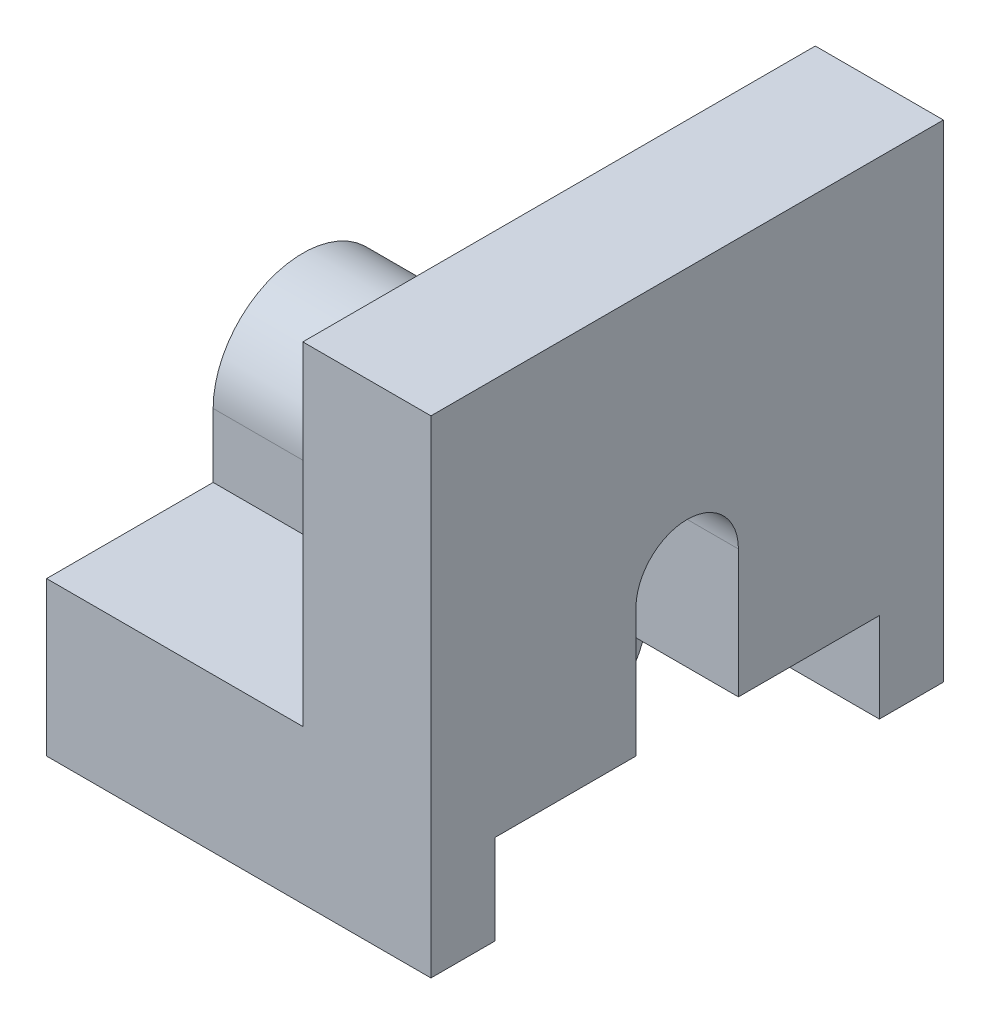
ISO-10303-21;
HEADER;
FILE_DESCRIPTION(('STEP AP214'),'2;1');
FILE_NAME('part.step','',(''),(''),'','','');
FILE_SCHEMA(('AUTOMOTIVE_DESIGN { 1 0 10303 214 1 1 1 1 }'));
ENDSEC;
DATA;
#1=APPLICATION_CONTEXT('core data for automotive mechanical design processes');
#2=APPLICATION_PROTOCOL_DEFINITION('international standard','automotive_design',2000,#1);
#3=PRODUCT_CONTEXT('',#1,'mechanical');
#4=PRODUCT('Part','Part','',(#3));
#5=PRODUCT_RELATED_PRODUCT_CATEGORY('part','',(#4));
#6=PRODUCT_DEFINITION_FORMATION('','',#4);
#7=PRODUCT_DEFINITION_CONTEXT('part definition',#1,'design');
#8=PRODUCT_DEFINITION('design','',#6,#7);
#9=PRODUCT_DEFINITION_SHAPE('','',#8);
#10=(LENGTH_UNIT() NAMED_UNIT(*) SI_UNIT(.MILLI.,.METRE.));
#11=(NAMED_UNIT(*) PLANE_ANGLE_UNIT() SI_UNIT($,.RADIAN.));
#12=(NAMED_UNIT(*) SI_UNIT($,.STERADIAN.) SOLID_ANGLE_UNIT());
#13=UNCERTAINTY_MEASURE_WITH_UNIT(LENGTH_MEASURE(1.E-05),#10,'distance_accuracy_value','');
#14=(GEOMETRIC_REPRESENTATION_CONTEXT(3) GLOBAL_UNCERTAINTY_ASSIGNED_CONTEXT((#13)) GLOBAL_UNIT_ASSIGNED_CONTEXT((#10,
#11,#12)) REPRESENTATION_CONTEXT('',''));
#15=CARTESIAN_POINT('',(0.,0.,0.));
#16=DIRECTION('',(0.,0.,1.));
#17=DIRECTION('',(1.,0.,0.));
#18=AXIS2_PLACEMENT_3D('',#15,#16,#17);
#19=CARTESIAN_POINT('',(20.,12.,40.));
#20=DIRECTION('',(1.,0.,0.));
#21=DIRECTION('',(0.,0.,-1.));
#22=AXIS2_PLACEMENT_3D('',#19,#20,#21);
#23=PLANE('',#22);
#24=DIRECTION('',(0.,-1.,0.));
#25=VECTOR('',#24,1.);
#26=CARTESIAN_POINT('',(20.,12.,17.5));
#27=LINE('',#26,#25);
#28=CARTESIAN_POINT('',(20.,38.,17.5));
#29=VERTEX_POINT('',#28);
#30=CARTESIAN_POINT('',(20.,23.538348415311,17.5));
#31=VERTEX_POINT('',#30);
#32=EDGE_CURVE('E53',#29,#31,#27,.T.);
#33=ORIENTED_EDGE('',*,*,#32,.F.);
#34=DIRECTION('',(0.,0.,-1.));
#35=VECTOR('',#34,1.);
#36=CARTESIAN_POINT('',(20.,38.,40.));
#37=LINE('',#36,#35);
#38=CARTESIAN_POINT('',(20.,38.,0.));
#39=VERTEX_POINT('',#38);
#40=EDGE_CURVE('E219',#29,#39,#37,.T.);
#41=ORIENTED_EDGE('',*,*,#40,.T.);
#42=DIRECTION('',(0.,-1.,0.));
#43=VECTOR('',#42,1.);
#44=CARTESIAN_POINT('',(20.,12.,0.));
#45=LINE('',#44,#43);
#46=CARTESIAN_POINT('',(20.,12.,0.));
#47=VERTEX_POINT('',#46);
#48=EDGE_CURVE('E283',#39,#47,#45,.T.);
#49=ORIENTED_EDGE('',*,*,#48,.T.);
#50=DIRECTION('',(0.,0.,-1.));
#51=VECTOR('',#50,1.);
#52=CARTESIAN_POINT('',(20.,12.,40.));
#53=LINE('',#52,#51);
#54=CARTESIAN_POINT('',(20.,12.,13.));
#55=VERTEX_POINT('',#54);
#56=EDGE_CURVE('E234',#55,#47,#53,.T.);
#57=ORIENTED_EDGE('',*,*,#56,.F.);
#58=DIRECTION('',(0.,-1.,0.));
#59=VECTOR('',#58,1.);
#60=CARTESIAN_POINT('',(20.,7.00000000000001,13.));
#61=LINE('',#60,#59);
#62=CARTESIAN_POINT('',(20.,17.,13.));
#63=VERTEX_POINT('',#62);
#64=EDGE_CURVE('E336',#63,#55,#61,.T.);
#65=ORIENTED_EDGE('',*,*,#64,.F.);
#66=CARTESIAN_POINT('',(20.,17.,20.));
#67=DIRECTION('',(-1.,0.,0.));
#68=DIRECTION('',(0.,0.,1.));
#69=AXIS2_PLACEMENT_3D('',#66,#67,#68);
#70=CIRCLE('',#69,7.);
#71=EDGE_CURVE('E63',#31,#63,#70,.T.);
#72=ORIENTED_EDGE('',*,*,#71,.F.);
#73=EDGE_LOOP('',(#33,#41,#49,#57,#65,#72));
#74=FACE_BOUND('',#73,.T.);
#75=ADVANCED_FACE('F39',(#74),#23,.F.);
#76=CARTESIAN_POINT('',(30.,7.,0.));
#77=DIRECTION('',(0.,1.,0.));
#78=DIRECTION('',(0.,0.,1.));
#79=AXIS2_PLACEMENT_3D('',#76,#77,#78);
#80=PLANE('',#79);
#81=DIRECTION('',(0.,0.,1.));
#82=VECTOR('',#81,1.);
#83=CARTESIAN_POINT('',(20.,7.,0.));
#84=LINE('',#83,#82);
#85=CARTESIAN_POINT('',(20.,7.,24.));
#86=VERTEX_POINT('',#85);
#87=CARTESIAN_POINT('',(20.,7.,27.));
#88=VERTEX_POINT('',#87);
#89=EDGE_CURVE('E43',#86,#88,#84,.T.);
#90=ORIENTED_EDGE('',*,*,#89,.F.);
#91=DIRECTION('',(-1.,0.,0.));
#92=VECTOR('',#91,1.);
#93=CARTESIAN_POINT('',(30.,7.,24.));
#94=LINE('',#93,#92);
#95=CARTESIAN_POINT('',(30.,7.,24.));
#96=VERTEX_POINT('',#95);
#97=EDGE_CURVE('E383',#96,#86,#94,.T.);
#98=ORIENTED_EDGE('',*,*,#97,.F.);
#99=DIRECTION('',(0.,0.,-1.));
#100=VECTOR('',#99,1.);
#101=CARTESIAN_POINT('',(30.,7.,0.));
#102=LINE('',#101,#100);
#103=CARTESIAN_POINT('',(30.,7.,35.));
#104=VERTEX_POINT('',#103);
#105=EDGE_CURVE('E322',#104,#96,#102,.T.);
#106=ORIENTED_EDGE('',*,*,#105,.F.);
#107=DIRECTION('',(-1.,0.,0.));
#108=VECTOR('',#107,1.);
#109=CARTESIAN_POINT('',(30.,7.,35.));
#110=LINE('',#109,#108);
#111=CARTESIAN_POINT('',(0.,7.,35.));
#112=VERTEX_POINT('',#111);
#113=EDGE_CURVE('E301',#104,#112,#110,.T.);
#114=ORIENTED_EDGE('',*,*,#113,.T.);
#115=DIRECTION('',(0.,0.,-1.));
#116=VECTOR('',#115,1.);
#117=CARTESIAN_POINT('',(0.,7.,0.));
#118=LINE('',#117,#116);
#119=CARTESIAN_POINT('',(0.,7.,27.));
#120=VERTEX_POINT('',#119);
#121=EDGE_CURVE('E314',#112,#120,#118,.T.);
#122=ORIENTED_EDGE('',*,*,#121,.T.);
#123=DIRECTION('',(-1.,0.,0.));
#124=VECTOR('',#123,1.);
#125=CARTESIAN_POINT('',(20.,7.00000000000001,27.));
#126=LINE('',#125,#124);
#127=EDGE_CURVE('E331',#88,#120,#126,.T.);
#128=ORIENTED_EDGE('',*,*,#127,.F.);
#129=EDGE_LOOP('',(#90,#98,#106,#114,#122,#128));
#130=FACE_BOUND('',#129,.T.);
#131=ADVANCED_FACE('F444',(#130),#80,.F.);
#132=CARTESIAN_POINT('',(30.,6.99999999999997,16.));
#133=VERTEX_POINT('',#132);
#134=CARTESIAN_POINT('',(30.,7.,5.));
#135=VERTEX_POINT('',#134);
#136=EDGE_CURVE('E330',#133,#135,#102,.T.);
#137=ORIENTED_EDGE('',*,*,#136,.F.);
#138=DIRECTION('',(-1.,0.,0.));
#139=VECTOR('',#138,1.);
#140=CARTESIAN_POINT('',(30.,6.99999999999997,16.));
#141=LINE('',#140,#139);
#142=CARTESIAN_POINT('',(20.,6.99999999999997,16.));
#143=VERTEX_POINT('',#142);
#144=EDGE_CURVE('E387',#133,#143,#141,.T.);
#145=ORIENTED_EDGE('',*,*,#144,.T.);
#146=CARTESIAN_POINT('',(20.,7.,13.));
#147=VERTEX_POINT('',#146);
#148=EDGE_CURVE('E11',#147,#143,#84,.T.);
#149=ORIENTED_EDGE('',*,*,#148,.F.);
#150=DIRECTION('',(-1.,0.,0.));
#151=VECTOR('',#150,1.);
#152=CARTESIAN_POINT('',(20.,7.00000000000001,13.));
#153=LINE('',#152,#151);
#154=CARTESIAN_POINT('',(0.,7.,13.));
#155=VERTEX_POINT('',#154);
#156=EDGE_CURVE('E334',#147,#155,#153,.T.);
#157=ORIENTED_EDGE('',*,*,#156,.T.);
#158=CARTESIAN_POINT('',(0.,7.,5.));
#159=VERTEX_POINT('',#158);
#160=EDGE_CURVE('E320',#155,#159,#118,.T.);
#161=ORIENTED_EDGE('',*,*,#160,.T.);
#162=DIRECTION('',(-1.,0.,0.));
#163=VECTOR('',#162,1.);
#164=CARTESIAN_POINT('',(30.,7.,5.));
#165=LINE('',#164,#163);
#166=EDGE_CURVE('E308',#135,#159,#165,.T.);
#167=ORIENTED_EDGE('',*,*,#166,.F.);
#168=EDGE_LOOP('',(#137,#145,#149,#157,#161,#167));
#169=FACE_BOUND('',#168,.T.);
#170=ADVANCED_FACE('F432',(#169),#80,.F.);
#171=CARTESIAN_POINT('',(0.,12.,40.));
#172=DIRECTION('',(0.,-1.,0.));
#173=DIRECTION('',(0.,0.,-1.));
#174=AXIS2_PLACEMENT_3D('',#171,#172,#173);
#175=PLANE('',#174);
#176=DIRECTION('',(0.,0.,-1.));
#177=VECTOR('',#176,1.);
#178=CARTESIAN_POINT('',(0.,12.,40.));
#179=LINE('',#178,#177);
#180=CARTESIAN_POINT('',(0.,12.,13.));
#181=VERTEX_POINT('',#180);
#182=CARTESIAN_POINT('',(0.,12.,0.));
#183=VERTEX_POINT('',#182);
#184=EDGE_CURVE('E269',#181,#183,#179,.T.);
#185=ORIENTED_EDGE('',*,*,#184,.F.);
#186=DIRECTION('',(1.,0.,0.));
#187=VECTOR('',#186,1.);
#188=CARTESIAN_POINT('',(0.,12.,13.));
#189=LINE('',#188,#187);
#190=EDGE_CURVE('E321',#181,#55,#189,.T.);
#191=ORIENTED_EDGE('',*,*,#190,.T.);
#192=ORIENTED_EDGE('',*,*,#56,.T.);
#193=DIRECTION('',(-1.,0.,0.));
#194=VECTOR('',#193,1.);
#195=CARTESIAN_POINT('',(0.,12.,0.));
#196=LINE('',#195,#194);
#197=EDGE_CURVE('E281',#47,#183,#196,.T.);
#198=ORIENTED_EDGE('',*,*,#197,.T.);
#199=EDGE_LOOP('',(#185,#191,#192,#198));
#200=FACE_BOUND('',#199,.T.);
#201=ADVANCED_FACE('F435',(#200),#175,.F.);
#202=CARTESIAN_POINT('',(0.,0.,40.));
#203=DIRECTION('',(0.,1.,0.));
#204=DIRECTION('',(0.,0.,1.));
#205=AXIS2_PLACEMENT_3D('',#202,#203,#204);
#206=PLANE('',#205);
#207=DIRECTION('',(-1.,0.,0.));
#208=VECTOR('',#207,1.);
#209=CARTESIAN_POINT('',(30.,0.,5.));
#210=LINE('',#209,#208);
#211=CARTESIAN_POINT('',(30.,0.,5.));
#212=VERTEX_POINT('',#211);
#213=CARTESIAN_POINT('',(0.,0.,5.));
#214=VERTEX_POINT('',#213);
#215=EDGE_CURVE('E258',#212,#214,#210,.T.);
#216=ORIENTED_EDGE('',*,*,#215,.T.);
#217=DIRECTION('',(0.,0.,-1.));
#218=VECTOR('',#217,1.);
#219=CARTESIAN_POINT('',(0.,0.,40.));
#220=LINE('',#219,#218);
#221=CARTESIAN_POINT('',(0.,0.,0.));
#222=VERTEX_POINT('',#221);
#223=EDGE_CURVE('E238',#214,#222,#220,.T.);
#224=ORIENTED_EDGE('',*,*,#223,.T.);
#225=DIRECTION('',(1.,0.,0.));
#226=VECTOR('',#225,1.);
#227=CARTESIAN_POINT('',(0.,0.,0.));
#228=LINE('',#227,#226);
#229=CARTESIAN_POINT('',(30.,0.,0.));
#230=VERTEX_POINT('',#229);
#231=EDGE_CURVE('E255',#222,#230,#228,.T.);
#232=ORIENTED_EDGE('',*,*,#231,.T.);
#233=DIRECTION('',(0.,0.,-1.));
#234=VECTOR('',#233,1.);
#235=CARTESIAN_POINT('',(30.,0.,40.));
#236=LINE('',#235,#234);
#237=EDGE_CURVE('E240',#212,#230,#236,.T.);
#238=ORIENTED_EDGE('',*,*,#237,.F.);
#239=EDGE_LOOP('',(#216,#224,#232,#238));
#240=FACE_BOUND('',#239,.T.);
#241=ADVANCED_FACE('F252',(#240),#206,.F.);
#242=CARTESIAN_POINT('',(0.,0.,40.));
#243=DIRECTION('',(1.,0.,0.));
#244=DIRECTION('',(0.,0.,-1.));
#245=AXIS2_PLACEMENT_3D('',#242,#243,#244);
#246=PLANE('',#245);
#247=CARTESIAN_POINT('',(0.,7.,20.));
#248=DIRECTION('',(-1.,0.,0.));
#249=DIRECTION('',(0.,0.,1.));
#250=AXIS2_PLACEMENT_3D('',#247,#248,#249);
#251=CIRCLE('',#250,7.);
#252=EDGE_CURVE('E355',#155,#120,#251,.T.);
#253=ORIENTED_EDGE('',*,*,#252,.T.);
#254=ORIENTED_EDGE('',*,*,#121,.F.);
#255=DIRECTION('',(0.,1.,0.));
#256=VECTOR('',#255,1.);
#257=CARTESIAN_POINT('',(0.,0.,35.));
#258=LINE('',#257,#256);
#259=CARTESIAN_POINT('',(0.,0.,35.));
#260=VERTEX_POINT('',#259);
#261=EDGE_CURVE('E318',#260,#112,#258,.T.);
#262=ORIENTED_EDGE('',*,*,#261,.F.);
#263=CARTESIAN_POINT('',(0.,0.,40.));
#264=VERTEX_POINT('',#263);
#265=EDGE_CURVE('E243',#264,#260,#220,.T.);
#266=ORIENTED_EDGE('',*,*,#265,.F.);
#267=DIRECTION('',(0.,-1.,0.));
#268=VECTOR('',#267,1.);
#269=CARTESIAN_POINT('',(0.,0.,40.));
#270=LINE('',#269,#268);
#271=CARTESIAN_POINT('',(0.,12.,40.));
#272=VERTEX_POINT('',#271);
#273=EDGE_CURVE('E284',#272,#264,#270,.T.);
#274=ORIENTED_EDGE('',*,*,#273,.F.);
#275=CARTESIAN_POINT('',(0.,12.,27.));
#276=VERTEX_POINT('',#275);
#277=EDGE_CURVE('E282',#272,#276,#179,.T.);
#278=ORIENTED_EDGE('',*,*,#277,.T.);
#279=DIRECTION('',(0.,1.,0.));
#280=VECTOR('',#279,1.);
#281=CARTESIAN_POINT('',(0.,7.00000000000001,27.));
#282=LINE('',#281,#280);
#283=CARTESIAN_POINT('',(0.,17.,27.));
#284=VERTEX_POINT('',#283);
#285=EDGE_CURVE('E348',#276,#284,#282,.T.);
#286=ORIENTED_EDGE('',*,*,#285,.T.);
#287=CARTESIAN_POINT('',(0.,17.,20.));
#288=DIRECTION('',(-1.,0.,0.));
#289=DIRECTION('',(0.,0.,1.));
#290=AXIS2_PLACEMENT_3D('',#287,#288,#289);
#291=CIRCLE('',#290,7.);
#292=CARTESIAN_POINT('',(0.,17.,13.));
#293=VERTEX_POINT('',#292);
#294=EDGE_CURVE('E350',#284,#293,#291,.T.);
#295=ORIENTED_EDGE('',*,*,#294,.T.);
#296=DIRECTION('',(0.,-1.,0.));
#297=VECTOR('',#296,1.);
#298=CARTESIAN_POINT('',(0.,7.00000000000001,13.));
#299=LINE('',#298,#297);
#300=EDGE_CURVE('E341',#293,#181,#299,.T.);
#301=ORIENTED_EDGE('',*,*,#300,.T.);
#302=ORIENTED_EDGE('',*,*,#184,.T.);
#303=DIRECTION('',(0.,-1.,0.));
#304=VECTOR('',#303,1.);
#305=CARTESIAN_POINT('',(0.,0.,0.));
#306=LINE('',#305,#304);
#307=EDGE_CURVE('E262',#183,#222,#306,.T.);
#308=ORIENTED_EDGE('',*,*,#307,.T.);
#309=ORIENTED_EDGE('',*,*,#223,.F.);
#310=DIRECTION('',(0.,1.,0.));
#311=VECTOR('',#310,1.);
#312=CARTESIAN_POINT('',(0.,0.,5.));
#313=LINE('',#312,#311);
#314=EDGE_CURVE('E313',#214,#159,#313,.T.);
#315=ORIENTED_EDGE('',*,*,#314,.T.);
#316=ORIENTED_EDGE('',*,*,#160,.F.);
#317=EDGE_LOOP('',(#253,#254,#262,#266,#274,#278,#286,#295,#301,#302,#308,#309,#315,#316));
#318=FACE_BOUND('',#317,.T.);
#319=DIRECTION('',(0.,1.,0.));
#320=VECTOR('',#319,1.);
#321=CARTESIAN_POINT('',(0.,7.,24.));
#322=LINE('',#321,#320);
#323=CARTESIAN_POINT('',(0.,7.,24.));
#324=VERTEX_POINT('',#323);
#325=CARTESIAN_POINT('',(0.,17.,24.));
#326=VERTEX_POINT('',#325);
#327=EDGE_CURVE('E379',#324,#326,#322,.T.);
#328=ORIENTED_EDGE('',*,*,#327,.F.);
#329=CARTESIAN_POINT('',(0.,7.,20.));
#330=DIRECTION('',(-1.,0.,0.));
#331=DIRECTION('',(0.,0.,1.));
#332=AXIS2_PLACEMENT_3D('',#329,#330,#331);
#333=CIRCLE('',#332,4.);
#334=CARTESIAN_POINT('',(0.,6.99999999999997,16.));
#335=VERTEX_POINT('',#334);
#336=EDGE_CURVE('E385',#335,#324,#333,.T.);
#337=ORIENTED_EDGE('',*,*,#336,.F.);
#338=DIRECTION('',(0.,-1.,0.));
#339=VECTOR('',#338,1.);
#340=CARTESIAN_POINT('',(0.,7.,16.));
#341=LINE('',#340,#339);
#342=CARTESIAN_POINT('',(0.,17.,16.));
#343=VERTEX_POINT('',#342);
#344=EDGE_CURVE('E374',#343,#335,#341,.T.);
#345=ORIENTED_EDGE('',*,*,#344,.F.);
#346=CARTESIAN_POINT('',(0.,17.,20.));
#347=DIRECTION('',(-1.,0.,0.));
#348=DIRECTION('',(0.,0.,1.));
#349=AXIS2_PLACEMENT_3D('',#346,#347,#348);
#350=CIRCLE('',#349,4.);
#351=EDGE_CURVE('E380',#326,#343,#350,.T.);
#352=ORIENTED_EDGE('',*,*,#351,.F.);
#353=EDGE_LOOP('',(#328,#337,#345,#352));
#354=FACE_BOUND('',#353,.T.);
#355=ADVANCED_FACE('F41',(#318,#354),#246,.F.);
#356=ORIENTED_EDGE('',*,*,#265,.T.);
#357=DIRECTION('',(-1.,0.,0.));
#358=VECTOR('',#357,1.);
#359=CARTESIAN_POINT('',(30.,0.,35.));
#360=LINE('',#359,#358);
#361=CARTESIAN_POINT('',(30.,0.,35.));
#362=VERTEX_POINT('',#361);
#363=EDGE_CURVE('E275',#362,#260,#360,.T.);
#364=ORIENTED_EDGE('',*,*,#363,.F.);
#365=CARTESIAN_POINT('',(30.,0.,40.));
#366=VERTEX_POINT('',#365);
#367=EDGE_CURVE('E236',#366,#362,#236,.T.);
#368=ORIENTED_EDGE('',*,*,#367,.F.);
#369=DIRECTION('',(1.,0.,0.));
#370=VECTOR('',#369,1.);
#371=CARTESIAN_POINT('',(0.,0.,40.));
#372=LINE('',#371,#370);
#373=EDGE_CURVE('E302',#264,#366,#372,.T.);
#374=ORIENTED_EDGE('',*,*,#373,.F.);
#375=EDGE_LOOP('',(#356,#364,#368,#374));
#376=FACE_BOUND('',#375,.T.);
#377=ADVANCED_FACE('F442',(#376),#206,.F.);
#378=CARTESIAN_POINT('',(30.,0.,40.));
#379=DIRECTION('',(-1.,0.,0.));
#380=DIRECTION('',(0.,0.,1.));
#381=AXIS2_PLACEMENT_3D('',#378,#379,#380);
#382=PLANE('',#381);
#383=CARTESIAN_POINT('',(30.,17.,20.));
#384=DIRECTION('',(-1.,0.,0.));
#385=DIRECTION('',(0.,0.,-1.));
#386=AXIS2_PLACEMENT_3D('',#383,#384,#385);
#387=CIRCLE('',#386,4.);
#388=CARTESIAN_POINT('',(30.,17.,24.));
#389=VERTEX_POINT('',#388);
#390=CARTESIAN_POINT('',(30.,17.,16.));
#391=VERTEX_POINT('',#390);
#392=EDGE_CURVE('E215',#389,#391,#387,.T.);
#393=ORIENTED_EDGE('',*,*,#392,.T.);
#394=DIRECTION('',(0.,-1.,0.));
#395=VECTOR('',#394,1.);
#396=CARTESIAN_POINT('',(30.,17.,16.));
#397=LINE('',#396,#395);
#398=EDGE_CURVE('E391',#391,#133,#397,.T.);
#399=ORIENTED_EDGE('',*,*,#398,.T.);
#400=ORIENTED_EDGE('',*,*,#136,.T.);
#401=DIRECTION('',(0.,1.,0.));
#402=VECTOR('',#401,1.);
#403=CARTESIAN_POINT('',(30.,0.,5.));
#404=LINE('',#403,#402);
#405=EDGE_CURVE('E307',#212,#135,#404,.T.);
#406=ORIENTED_EDGE('',*,*,#405,.F.);
#407=ORIENTED_EDGE('',*,*,#237,.T.);
#408=DIRECTION('',(0.,1.,0.));
#409=VECTOR('',#408,1.);
#410=CARTESIAN_POINT('',(30.,0.,0.));
#411=LINE('',#410,#409);
#412=CARTESIAN_POINT('',(30.,38.,0.));
#413=VERTEX_POINT('',#412);
#414=EDGE_CURVE('E266',#230,#413,#411,.T.);
#415=ORIENTED_EDGE('',*,*,#414,.T.);
#416=DIRECTION('',(0.,0.,-1.));
#417=VECTOR('',#416,1.);
#418=CARTESIAN_POINT('',(30.,38.,40.));
#419=LINE('',#418,#417);
#420=CARTESIAN_POINT('',(30.,38.,40.));
#421=VERTEX_POINT('',#420);
#422=EDGE_CURVE('E227',#421,#413,#419,.T.);
#423=ORIENTED_EDGE('',*,*,#422,.F.);
#424=DIRECTION('',(0.,1.,0.));
#425=VECTOR('',#424,1.);
#426=CARTESIAN_POINT('',(30.,0.,40.));
#427=LINE('',#426,#425);
#428=EDGE_CURVE('E300',#366,#421,#427,.T.);
#429=ORIENTED_EDGE('',*,*,#428,.F.);
#430=ORIENTED_EDGE('',*,*,#367,.T.);
#431=DIRECTION('',(0.,1.,0.));
#432=VECTOR('',#431,1.);
#433=CARTESIAN_POINT('',(30.,0.,35.));
#434=LINE('',#433,#432);
#435=EDGE_CURVE('E311',#362,#104,#434,.T.);
#436=ORIENTED_EDGE('',*,*,#435,.T.);
#437=ORIENTED_EDGE('',*,*,#105,.T.);
#438=DIRECTION('',(0.,1.,0.));
#439=VECTOR('',#438,1.);
#440=CARTESIAN_POINT('',(30.,7.,24.));
#441=LINE('',#440,#439);
#442=EDGE_CURVE('E389',#96,#389,#441,.T.);
#443=ORIENTED_EDGE('',*,*,#442,.T.);
#444=EDGE_LOOP('',(#393,#399,#400,#406,#407,#415,#423,#429,#430,#436,#437,#443));
#445=FACE_BOUND('',#444,.T.);
#446=ADVANCED_FACE('F421',(#445),#382,.F.);
#447=CARTESIAN_POINT('',(30.,38.,40.));
#448=DIRECTION('',(0.,-1.,0.));
#449=DIRECTION('',(0.,0.,-1.));
#450=AXIS2_PLACEMENT_3D('',#447,#448,#449);
#451=PLANE('',#450);
#452=ORIENTED_EDGE('',*,*,#422,.T.);
#453=DIRECTION('',(-1.,0.,0.));
#454=VECTOR('',#453,1.);
#455=CARTESIAN_POINT('',(30.,38.,0.));
#456=LINE('',#455,#454);
#457=EDGE_CURVE('E223',#413,#39,#456,.T.);
#458=ORIENTED_EDGE('',*,*,#457,.T.);
#459=ORIENTED_EDGE('',*,*,#40,.F.);
#460=DIRECTION('',(0.,0.,1.));
#461=VECTOR('',#460,1.);
#462=CARTESIAN_POINT('',(20.,38.,40.));
#463=LINE('',#462,#461);
#464=CARTESIAN_POINT('',(20.,38.,22.5));
#465=VERTEX_POINT('',#464);
#466=EDGE_CURVE('E205',#29,#465,#463,.T.);
#467=ORIENTED_EDGE('',*,*,#466,.T.);
#468=CARTESIAN_POINT('',(20.,38.,40.));
#469=VERTEX_POINT('',#468);
#470=EDGE_CURVE('E230',#469,#465,#37,.T.);
#471=ORIENTED_EDGE('',*,*,#470,.F.);
#472=DIRECTION('',(-1.,0.,0.));
#473=VECTOR('',#472,1.);
#474=CARTESIAN_POINT('',(30.,38.,40.));
#475=LINE('',#474,#473);
#476=EDGE_CURVE('E294',#421,#469,#475,.T.);
#477=ORIENTED_EDGE('',*,*,#476,.F.);
#478=EDGE_LOOP('',(#452,#458,#459,#467,#471,#477));
#479=FACE_BOUND('',#478,.T.);
#480=ADVANCED_FACE('F224',(#479),#451,.F.);
#481=ORIENTED_EDGE('',*,*,#470,.T.);
#482=DIRECTION('',(0.,-1.,0.));
#483=VECTOR('',#482,1.);
#484=CARTESIAN_POINT('',(20.,12.,22.5));
#485=LINE('',#484,#483);
#486=CARTESIAN_POINT('',(20.,23.538348415311,22.5));
#487=VERTEX_POINT('',#486);
#488=EDGE_CURVE('E398',#465,#487,#485,.T.);
#489=ORIENTED_EDGE('',*,*,#488,.T.);
#490=CARTESIAN_POINT('',(20.,17.,27.));
#491=VERTEX_POINT('',#490);
#492=EDGE_CURVE('E359',#491,#487,#70,.T.);
#493=ORIENTED_EDGE('',*,*,#492,.F.);
#494=DIRECTION('',(0.,1.,0.));
#495=VECTOR('',#494,1.);
#496=CARTESIAN_POINT('',(20.,7.00000000000001,27.));
#497=LINE('',#496,#495);
#498=CARTESIAN_POINT('',(20.,12.,27.));
#499=VERTEX_POINT('',#498);
#500=EDGE_CURVE('E358',#499,#491,#497,.T.);
#501=ORIENTED_EDGE('',*,*,#500,.F.);
#502=CARTESIAN_POINT('',(20.,12.,40.));
#503=VERTEX_POINT('',#502);
#504=EDGE_CURVE('E226',#503,#499,#53,.T.);
#505=ORIENTED_EDGE('',*,*,#504,.F.);
#506=DIRECTION('',(0.,-1.,0.));
#507=VECTOR('',#506,1.);
#508=CARTESIAN_POINT('',(20.,12.,40.));
#509=LINE('',#508,#507);
#510=EDGE_CURVE('E288',#469,#503,#509,.T.);
#511=ORIENTED_EDGE('',*,*,#510,.F.);
#512=EDGE_LOOP('',(#481,#489,#493,#501,#505,#511));
#513=FACE_BOUND('',#512,.T.);
#514=ADVANCED_FACE('F412',(#513),#23,.F.);
#515=ORIENTED_EDGE('',*,*,#504,.T.);
#516=DIRECTION('',(-1.,0.,0.));
#517=VECTOR('',#516,1.);
#518=CARTESIAN_POINT('',(0.,12.,27.));
#519=LINE('',#518,#517);
#520=EDGE_CURVE('E332',#499,#276,#519,.T.);
#521=ORIENTED_EDGE('',*,*,#520,.T.);
#522=ORIENTED_EDGE('',*,*,#277,.F.);
#523=DIRECTION('',(-1.,0.,0.));
#524=VECTOR('',#523,1.);
#525=CARTESIAN_POINT('',(0.,12.,40.));
#526=LINE('',#525,#524);
#527=EDGE_CURVE('E277',#503,#272,#526,.T.);
#528=ORIENTED_EDGE('',*,*,#527,.F.);
#529=EDGE_LOOP('',(#515,#521,#522,#528));
#530=FACE_BOUND('',#529,.T.);
#531=ADVANCED_FACE('F418',(#530),#175,.F.);
#532=CARTESIAN_POINT('',(0.,0.,40.));
#533=DIRECTION('',(0.,0.,-1.));
#534=DIRECTION('',(-1.,0.,0.));
#535=AXIS2_PLACEMENT_3D('',#532,#533,#534);
#536=PLANE('',#535);
#537=ORIENTED_EDGE('',*,*,#273,.T.);
#538=ORIENTED_EDGE('',*,*,#373,.T.);
#539=ORIENTED_EDGE('',*,*,#428,.T.);
#540=ORIENTED_EDGE('',*,*,#476,.T.);
#541=ORIENTED_EDGE('',*,*,#510,.T.);
#542=ORIENTED_EDGE('',*,*,#527,.T.);
#543=EDGE_LOOP('',(#537,#538,#539,#540,#541,#542));
#544=FACE_BOUND('',#543,.T.);
#545=ADVANCED_FACE('F420',(#544),#536,.F.);
#546=CARTESIAN_POINT('',(0.,0.,0.));
#547=DIRECTION('',(0.,0.,-1.));
#548=DIRECTION('',(-1.,0.,0.));
#549=AXIS2_PLACEMENT_3D('',#546,#547,#548);
#550=PLANE('',#549);
#551=ORIENTED_EDGE('',*,*,#307,.F.);
#552=ORIENTED_EDGE('',*,*,#197,.F.);
#553=ORIENTED_EDGE('',*,*,#48,.F.);
#554=ORIENTED_EDGE('',*,*,#457,.F.);
#555=ORIENTED_EDGE('',*,*,#414,.F.);
#556=ORIENTED_EDGE('',*,*,#231,.F.);
#557=EDGE_LOOP('',(#551,#552,#553,#554,#555,#556));
#558=FACE_BOUND('',#557,.T.);
#559=ADVANCED_FACE('F265',(#558),#550,.T.);
#560=CARTESIAN_POINT('',(30.,0.,35.));
#561=DIRECTION('',(0.,0.,1.));
#562=DIRECTION('',(1.,0.,0.));
#563=AXIS2_PLACEMENT_3D('',#560,#561,#562);
#564=PLANE('',#563);
#565=ORIENTED_EDGE('',*,*,#261,.T.);
#566=ORIENTED_EDGE('',*,*,#113,.F.);
#567=ORIENTED_EDGE('',*,*,#435,.F.);
#568=ORIENTED_EDGE('',*,*,#363,.T.);
#569=EDGE_LOOP('',(#565,#566,#567,#568));
#570=FACE_BOUND('',#569,.T.);
#571=ADVANCED_FACE('F514',(#570),#564,.F.);
#572=CARTESIAN_POINT('',(30.,0.,5.));
#573=DIRECTION('',(0.,0.,1.));
#574=DIRECTION('',(1.,0.,0.));
#575=AXIS2_PLACEMENT_3D('',#572,#573,#574);
#576=PLANE('',#575);
#577=ORIENTED_EDGE('',*,*,#314,.F.);
#578=ORIENTED_EDGE('',*,*,#215,.F.);
#579=ORIENTED_EDGE('',*,*,#405,.T.);
#580=ORIENTED_EDGE('',*,*,#166,.T.);
#581=EDGE_LOOP('',(#577,#578,#579,#580));
#582=FACE_BOUND('',#581,.T.);
#583=ADVANCED_FACE('F528',(#582),#576,.T.);
#584=CARTESIAN_POINT('',(20.,7.,20.));
#585=DIRECTION('',(-1.,0.,0.));
#586=DIRECTION('',(0.,0.,1.));
#587=AXIS2_PLACEMENT_3D('',#584,#585,#586);
#588=CYLINDRICAL_SURFACE('',#587,4.);
#589=DIRECTION('',(-1.,0.,0.));
#590=VECTOR('',#589,1.);
#591=CARTESIAN_POINT('',(20.,7.,24.));
#592=LINE('',#591,#590);
#593=EDGE_CURVE('E365',#86,#324,#592,.T.);
#594=ORIENTED_EDGE('',*,*,#593,.F.);
#595=CARTESIAN_POINT('',(20.,7.,20.));
#596=DIRECTION('',(-1.,0.,0.));
#597=DIRECTION('',(0.,0.,1.));
#598=AXIS2_PLACEMENT_3D('',#595,#596,#597);
#599=CIRCLE('',#598,4.);
#600=EDGE_CURVE('E366',#143,#86,#599,.T.);
#601=ORIENTED_EDGE('',*,*,#600,.F.);
#602=DIRECTION('',(-1.,0.,0.));
#603=VECTOR('',#602,1.);
#604=CARTESIAN_POINT('',(20.,7.,16.));
#605=LINE('',#604,#603);
#606=EDGE_CURVE('E354',#143,#335,#605,.T.);
#607=ORIENTED_EDGE('',*,*,#606,.T.);
#608=ORIENTED_EDGE('',*,*,#336,.T.);
#609=EDGE_LOOP('',(#594,#601,#607,#608));
#610=FACE_BOUND('',#609,.T.);
#611=ADVANCED_FACE('F534',(#610),#588,.F.);
#612=CARTESIAN_POINT('',(20.,7.,20.));
#613=DIRECTION('',(-1.,0.,0.));
#614=DIRECTION('',(0.,0.,1.));
#615=AXIS2_PLACEMENT_3D('',#612,#613,#614);
#616=PLANE('',#615);
#617=ORIENTED_EDGE('',*,*,#89,.T.);
#618=CARTESIAN_POINT('',(20.,7.,20.));
#619=DIRECTION('',(-1.,0.,0.));
#620=DIRECTION('',(0.,0.,1.));
#621=AXIS2_PLACEMENT_3D('',#618,#619,#620);
#622=CIRCLE('',#621,7.);
#623=EDGE_CURVE('E347',#147,#88,#622,.T.);
#624=ORIENTED_EDGE('',*,*,#623,.F.);
#625=ORIENTED_EDGE('',*,*,#148,.T.);
#626=ORIENTED_EDGE('',*,*,#600,.T.);
#627=EDGE_LOOP('',(#617,#624,#625,#626));
#628=FACE_BOUND('',#627,.T.);
#629=ADVANCED_FACE('F544',(#628),#616,.F.);
#630=CARTESIAN_POINT('',(20.,7.,20.));
#631=DIRECTION('',(-1.,0.,0.));
#632=DIRECTION('',(0.,0.,1.));
#633=AXIS2_PLACEMENT_3D('',#630,#631,#632);
#634=CYLINDRICAL_SURFACE('',#633,7.);
#635=ORIENTED_EDGE('',*,*,#127,.T.);
#636=ORIENTED_EDGE('',*,*,#252,.F.);
#637=ORIENTED_EDGE('',*,*,#156,.F.);
#638=ORIENTED_EDGE('',*,*,#623,.T.);
#639=EDGE_LOOP('',(#635,#636,#637,#638));
#640=FACE_BOUND('',#639,.T.);
#641=ADVANCED_FACE('F551',(#640),#634,.T.);
#642=CARTESIAN_POINT('',(20.,7.00000000000001,13.));
#643=DIRECTION('',(0.,0.,-1.));
#644=DIRECTION('',(0.,1.,0.));
#645=AXIS2_PLACEMENT_3D('',#642,#643,#644);
#646=PLANE('',#645);
#647=ORIENTED_EDGE('',*,*,#190,.F.);
#648=ORIENTED_EDGE('',*,*,#300,.F.);
#649=DIRECTION('',(-1.,0.,0.));
#650=VECTOR('',#649,1.);
#651=CARTESIAN_POINT('',(20.,17.,13.));
#652=LINE('',#651,#650);
#653=EDGE_CURVE('E342',#63,#293,#652,.T.);
#654=ORIENTED_EDGE('',*,*,#653,.F.);
#655=ORIENTED_EDGE('',*,*,#64,.T.);
#656=EDGE_LOOP('',(#647,#648,#654,#655));
#657=FACE_BOUND('',#656,.T.);
#658=ADVANCED_FACE('F429',(#657),#646,.T.);
#659=CARTESIAN_POINT('',(20.,7.00000000000001,27.));
#660=DIRECTION('',(0.,0.,1.));
#661=DIRECTION('',(0.,-1.,0.));
#662=AXIS2_PLACEMENT_3D('',#659,#660,#661);
#663=PLANE('',#662);
#664=ORIENTED_EDGE('',*,*,#520,.F.);
#665=ORIENTED_EDGE('',*,*,#500,.T.);
#666=DIRECTION('',(-1.,0.,0.));
#667=VECTOR('',#666,1.);
#668=CARTESIAN_POINT('',(20.,17.,27.));
#669=LINE('',#668,#667);
#670=EDGE_CURVE('E340',#491,#284,#669,.T.);
#671=ORIENTED_EDGE('',*,*,#670,.T.);
#672=ORIENTED_EDGE('',*,*,#285,.F.);
#673=EDGE_LOOP('',(#664,#665,#671,#672));
#674=FACE_BOUND('',#673,.T.);
#675=ADVANCED_FACE('F411',(#674),#663,.T.);
#676=CARTESIAN_POINT('',(20.,7.,16.));
#677=DIRECTION('',(0.,0.,-1.));
#678=DIRECTION('',(-1.,0.,0.));
#679=AXIS2_PLACEMENT_3D('',#676,#677,#678);
#680=PLANE('',#679);
#681=ORIENTED_EDGE('',*,*,#344,.T.);
#682=ORIENTED_EDGE('',*,*,#606,.F.);
#683=ORIENTED_EDGE('',*,*,#144,.F.);
#684=ORIENTED_EDGE('',*,*,#398,.F.);
#685=DIRECTION('',(-1.,0.,0.));
#686=VECTOR('',#685,1.);
#687=CARTESIAN_POINT('',(20.,17.,16.));
#688=LINE('',#687,#686);
#689=EDGE_CURVE('E371',#391,#343,#688,.T.);
#690=ORIENTED_EDGE('',*,*,#689,.T.);
#691=EDGE_LOOP('',(#681,#682,#683,#684,#690));
#692=FACE_BOUND('',#691,.T.);
#693=ADVANCED_FACE('F579',(#692),#680,.F.);
#694=CARTESIAN_POINT('',(20.,7.,24.));
#695=DIRECTION('',(0.,0.,1.));
#696=DIRECTION('',(1.,0.,0.));
#697=AXIS2_PLACEMENT_3D('',#694,#695,#696);
#698=PLANE('',#697);
#699=DIRECTION('',(-1.,0.,0.));
#700=VECTOR('',#699,1.);
#701=CARTESIAN_POINT('',(20.,17.,24.));
#702=LINE('',#701,#700);
#703=EDGE_CURVE('E370',#389,#326,#702,.T.);
#704=ORIENTED_EDGE('',*,*,#703,.F.);
#705=ORIENTED_EDGE('',*,*,#442,.F.);
#706=ORIENTED_EDGE('',*,*,#97,.T.);
#707=ORIENTED_EDGE('',*,*,#593,.T.);
#708=ORIENTED_EDGE('',*,*,#327,.T.);
#709=EDGE_LOOP('',(#704,#705,#706,#707,#708));
#710=FACE_BOUND('',#709,.T.);
#711=ADVANCED_FACE('F584',(#710),#698,.F.);
#712=CARTESIAN_POINT('',(20.,17.,20.));
#713=DIRECTION('',(-1.,0.,0.));
#714=DIRECTION('',(0.,0.,1.));
#715=AXIS2_PLACEMENT_3D('',#712,#713,#714);
#716=CYLINDRICAL_SURFACE('',#715,7.);
#717=DIRECTION('',(-1.,0.,0.));
#718=VECTOR('',#717,1.);
#719=CARTESIAN_POINT('',(20.,23.538348415311,22.5));
#720=LINE('',#719,#718);
#721=CARTESIAN_POINT('',(5.53834841531107,23.538348415311,22.5));
#722=VERTEX_POINT('',#721);
#723=EDGE_CURVE('E400',#722,#487,#720,.F.);
#724=ORIENTED_EDGE('',*,*,#723,.F.);
#725=CARTESIAN_POINT('',(-0.999999999999914,17.,20.));
#726=DIRECTION('',(-0.707106781186549,0.707106781186546,0.));
#727=DIRECTION('',(-0.707106781186546,-0.707106781186549,0.));
#728=AXIS2_PLACEMENT_3D('',#725,#726,#727);
#729=ELLIPSE('',#728,9.89949493661164,7.);
#730=CARTESIAN_POINT('',(5.53834841531107,23.538348415311,17.5));
#731=VERTEX_POINT('',#730);
#732=EDGE_CURVE('E213',#731,#722,#729,.F.);
#733=ORIENTED_EDGE('',*,*,#732,.F.);
#734=DIRECTION('',(-1.,0.,0.));
#735=VECTOR('',#734,1.);
#736=CARTESIAN_POINT('',(20.,23.538348415311,17.5));
#737=LINE('',#736,#735);
#738=EDGE_CURVE('E216',#731,#31,#737,.F.);
#739=ORIENTED_EDGE('',*,*,#738,.T.);
#740=ORIENTED_EDGE('',*,*,#71,.T.);
#741=ORIENTED_EDGE('',*,*,#653,.T.);
#742=ORIENTED_EDGE('',*,*,#294,.F.);
#743=ORIENTED_EDGE('',*,*,#670,.F.);
#744=ORIENTED_EDGE('',*,*,#492,.T.);
#745=EDGE_LOOP('',(#724,#733,#739,#740,#741,#742,#743,#744));
#746=FACE_BOUND('',#745,.T.);
#747=ADVANCED_FACE('F410',(#746),#716,.T.);
#748=CARTESIAN_POINT('',(20.,17.,20.));
#749=DIRECTION('',(-1.,0.,0.));
#750=DIRECTION('',(0.,0.,1.));
#751=AXIS2_PLACEMENT_3D('',#748,#749,#750);
#752=CYLINDRICAL_SURFACE('',#751,4.);
#753=ORIENTED_EDGE('',*,*,#689,.F.);
#754=ORIENTED_EDGE('',*,*,#392,.F.);
#755=ORIENTED_EDGE('',*,*,#703,.T.);
#756=ORIENTED_EDGE('',*,*,#351,.T.);
#757=EDGE_LOOP('',(#753,#754,#755,#756));
#758=FACE_BOUND('',#757,.T.);
#759=ADVANCED_FACE('F602',(#758),#752,.F.);
#760=CARTESIAN_POINT('',(20.,38.,20.));
#761=DIRECTION('',(-0.707106781186549,0.707106781186546,0.));
#762=DIRECTION('',(-0.707106781186546,-0.707106781186549,0.));
#763=AXIS2_PLACEMENT_3D('',#760,#761,#762);
#764=PLANE('',#763);
#765=ORIENTED_EDGE('',*,*,#466,.F.);
#766=DIRECTION('',(-0.707106781186546,-0.707106781186549,0.));
#767=VECTOR('',#766,1.);
#768=CARTESIAN_POINT('',(20.,38.,17.5));
#769=LINE('',#768,#767);
#770=EDGE_CURVE('E204',#29,#731,#769,.T.);
#771=ORIENTED_EDGE('',*,*,#770,.T.);
#772=ORIENTED_EDGE('',*,*,#732,.T.);
#773=DIRECTION('',(-0.707106781186546,-0.707106781186549,0.));
#774=VECTOR('',#773,1.);
#775=CARTESIAN_POINT('',(20.,38.,22.5));
#776=LINE('',#775,#774);
#777=EDGE_CURVE('E210',#465,#722,#776,.T.);
#778=ORIENTED_EDGE('',*,*,#777,.F.);
#779=EDGE_LOOP('',(#765,#771,#772,#778));
#780=FACE_BOUND('',#779,.T.);
#781=ADVANCED_FACE('F201',(#780),#764,.T.);
#782=CARTESIAN_POINT('',(15.,19.,22.5));
#783=DIRECTION('',(0.,0.,1.));
#784=DIRECTION('',(1.,0.,0.));
#785=AXIS2_PLACEMENT_3D('',#782,#783,#784);
#786=PLANE('',#785);
#787=ORIENTED_EDGE('',*,*,#777,.T.);
#788=ORIENTED_EDGE('',*,*,#723,.T.);
#789=ORIENTED_EDGE('',*,*,#488,.F.);
#790=EDGE_LOOP('',(#787,#788,#789));
#791=FACE_BOUND('',#790,.T.);
#792=ADVANCED_FACE('F408',(#791),#786,.T.);
#793=CARTESIAN_POINT('',(15.,19.,17.5));
#794=DIRECTION('',(0.,0.,1.));
#795=DIRECTION('',(1.,0.,0.));
#796=AXIS2_PLACEMENT_3D('',#793,#794,#795);
#797=PLANE('',#796);
#798=ORIENTED_EDGE('',*,*,#738,.F.);
#799=ORIENTED_EDGE('',*,*,#770,.F.);
#800=ORIENTED_EDGE('',*,*,#32,.T.);
#801=EDGE_LOOP('',(#798,#799,#800));
#802=FACE_BOUND('',#801,.T.);
#803=ADVANCED_FACE('F214',(#802),#797,.F.);
#804=CLOSED_SHELL('',(#75,#131,#170,#201,#241,#355,#377,#446,#480,#514,#531,#545,#559,#571,#583,
#611,#629,#641,#658,#675,#693,#711,#747,#759,#781,#792,#803));
#805=MANIFOLD_SOLID_BREP('B2',#804);
#806=ADVANCED_BREP_SHAPE_REPRESENTATION('',(#18,#805),#14);
#807=SHAPE_DEFINITION_REPRESENTATION(#9,#806);
ENDSEC;
END-ISO-10303-21;
